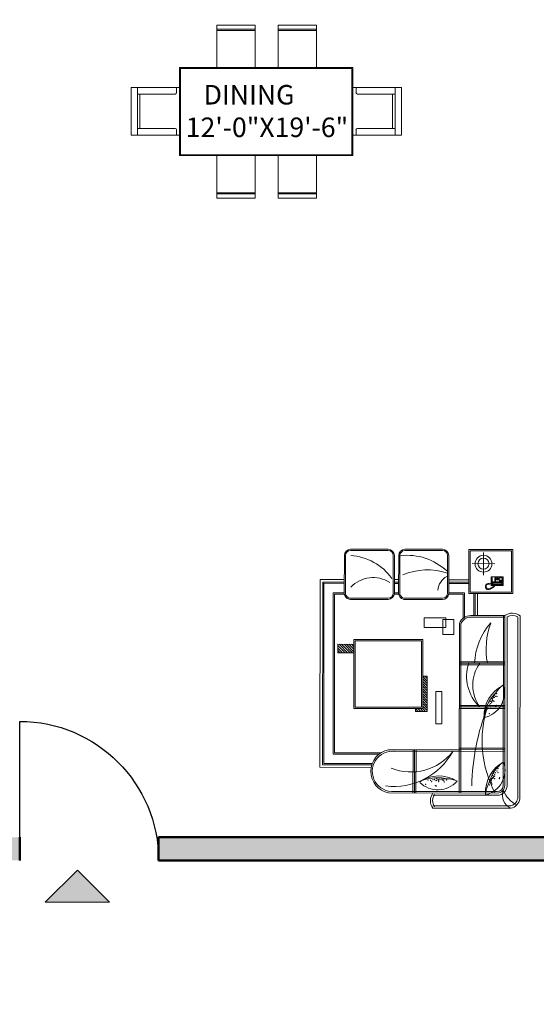
# Model space of a CAD drawing. Units: inches. Extents: x -7 to 1228, y -146 to 1091.
# Tile 49 of 88: x 242 to 376, y 531 to 786. Entities that reach past the tile are written whole.
import ezdxf

# ---------------------------------------------------------------- set-up
doc = ezdxf.new("R2010")
doc.units = ezdxf.units.IN
for name, color, linetype, lineweight in [('A-ANNO-SYMB', 30, 'Continuous', 18), ('A-AREA-IDEN', 7, 'Continuous', 18), ('A-DOOR', 4, 'Continuous', 25), ('A-FURN', 8, 'Continuous', 18), ('A-WALL', 7, 'Continuous', 50), ('A-WALL-PATT', 251, 'Continuous', 13)]:
    doc.layers.add(name, color=color, linetype=linetype, lineweight=lineweight)
doc.styles.get("Standard").update_dxf_attribs({"font": 'arial.ttf'})

# ---------------------------------------------------------------- blocks, each defined once
blk = doc.blocks.new('A$C317A697B')
for p, q in [((-116, 441), (-514, 441)), ((-514, 441), (-514, 0)), ((-116, 0), (-116, 441)), ((523, 441), (125, 441)), ((125, 441), (125, 0)), ((523, 0), (523, 441)), ((-116, 398), (-514, 398)), ((-116, 385), (-514, 385)), ((523, 398), (125, 398)), ((523, 385), (125, 385)), ((-899, -912), (-899, 0)), ((-899, 0), (899, 0)), ((899, 0), (899, -912)), ((-889, -902), (-889, -10)), ((-889, -10), (889, -10)), ((889, -10), (889, -902)), ((-899, -205), (-1402, -205)), ((-1402, -205), (-1402, -699)), ((-1336, -205), (-1336, -699)), ((-946, -274), (-1336, -274)), ((-1311, -274), (-1311, -630)), ((-932, -205), (-932, -259)), ((899, -205), (1402, -205)), ((932, -205), (932, -259)), ((946, -274), (1336, -274)), ((1311, -274), (1311, -630)), ((1336, -205), (1336, -699)), ((1402, -205), (1402, -699)), ((-1402, -699), (-899, -699)), ((-946, -630), (-1336, -630)), ((-932, -699), (-932, -645)), ((1402, -699), (899, -699)), ((932, -699), (932, -645)), ((946, -630), (1336, -630)), ((899, -912), (-899, -912)), ((889, -902), (-889, -902)), ((-514, -1353), (-514, -912)), ((-116, -912), (-116, -1353)), ((125, -1353), (125, -912)), ((523, -912), (523, -1353)), ((-116, -1297), (-514, -1297)), ((-116, -1309), (-514, -1309)), ((523, -1297), (125, -1297)), ((523, -1309), (125, -1309)), ((-116, -1353), (-514, -1353)), ((523, -1353), (125, -1353))]:
    blk.add_line(p, q)
for centre, start, end in [((-946, -259), 270, 0), ((946, -259), 180, 270), ((-946, -645), 0, 90), ((946, -645), 90, 180)]:
    blk.add_arc(centre, 14.7, start, end)
blk = doc.blocks.new('A$C327A19D4')
for p, q in [((1059, 3191), (3976, 3191)), ((1078, 3155), (3976, 3155)), ((703, 3073), (3, 3073)), ((3, 3073), (3, 2373)), ((683, 3053), (23, 3053)), ((23, 3053), (23, 2393)), ((683, 2393), (683, 3053)), ((703, 2373), (703, 3073)), ((1076, 2985), (3780, 2985)), ((4090, 3043), (4090, 1800)), ((4126, 3043), (4126, 1800)), ((1056, 2949), (3763, 2949)), ((1056, 2403), (1056, 2949)), ((1056, 2925), (3763, 2925)), ((1080, 2403), (1080, 2949)), ((1791, 2223), (1791, 2949)), ((1815, 2465), (1815, 2949)), ((1815, 2223), (1815, 2872)), ((1815, 2223), (1815, 2872)), ((1815, 2465), (1815, 2872)), ((1815, 2465), (1815, 2872)), ((1839, 2223), (1839, 2949)), ((2487, 2223), (2487, 2949)), ((2511, 2223), (2511, 2949)), ((2535, 2223), (2535, 2949)), ((3169, 2223), (3169, 2949)), ((3193, 2465), (3193, 2949)), ((3193, 2223), (3193, 2872)), ((3193, 2223), (3193, 2872)), ((3193, 2465), (3193, 2872)), ((3193, 2465), (3193, 2872)), ((3221, 1195), (3221, 2949)), ((3860, 2828), (3860, 1185)), ((3884, 2828), (3884, 1095)), ((3920, 2867), (3920, 1802)), ((231, 2784), (227, 2425)), ((49, 2607), (409, 2603)), ((703, 2512), (1056, 2512)), ((3, 2373), (703, 2373)), ((23, 2393), (683, 2393)), ((484, 2052), (484, 2373)), ((524, 2052), (524, 2373)), ((544, 2052), (544, 2373)), ((703, 2472), (1056, 2472)), ((703, 2452), (1056, 2452)), ((694, 2052), (694, 2302)), ((694, 2302), (1084, 2302)), ((714, 2051), (714, 2282)), ((714, 2282), (1098, 2282)), ((3884, 2247), (1184, 2247)), ((3884, 2223), (1184, 2223)), ((3195, 2235), (3195, 1095)), ((1119, 2135), (1357, 2135)), ((1119, 1958), (1119, 2135)), ((1357, 2135), (1357, 1958)), ((1092, 2007), (1244, 2007)), ((1092, 1659), (1092, 2007)), ((1357, 1958), (1119, 1958)), ((1244, 2007), (1244, 1659)), ((2265, 1945), (2780, 1945)), ((2265, 1845), (2265, 1945)), ((2780, 1945), (2780, 1845)), ((2780, 1845), (2265, 1845)), ((1244, 1659), (1092, 1659)), ((2539, 1638), (1439, 1638)), ((1439, 1638), (1439, 538)), ((2519, 1618), (1459, 1618)), ((1459, 1618), (1459, 558)), ((2023, 1638), (2023, 1711)), ((2023, 1711), (2585, 1711)), ((2519, 558), (2519, 1618)), ((2539, 538), (2539, 1638)), ((2585, 1711), (2585, 1522)), ((2585, 1522), (2539, 1522)), ((3884, 1532), (3195, 1532)), ((3884, 1508), (3195, 1508)), ((3884, 1484), (3195, 1484)), ((484, 1185), (484, 1252)), ((524, 1185), (524, 1252)), ((544, 1185), (544, 1252)), ((694, 1185), (694, 1252)), ((714, 1184), (714, 1253)), ((3247, 967), (3247, 230)), ((3267, 940), (3267, 210)), ((3417, 832), (3417, 60)), ((3437, 825), (3437, 40)), ((3477, 816), (3477, 0)), ((1439, 538), (2539, 538)), ((1459, 558), (2519, 558)), ((1516, 538), (1651, 538)), ((1516, 285), (1516, 538)), ((1651, 538), (1651, 285)), ((484, 0), (484, 385)), ((524, 40), (524, 385)), ((544, 60), (544, 385)), ((694, 210), (694, 385)), ((714, 230), (714, 386)), ((3267, 210), (694, 210)), ((3247, 230), (714, 230)), ((1651, 285), (1516, 285)), ((3437, 40), (524, 40)), ((3417, 60), (544, 60)), ((3477, 0), (484, 0))]:
    blk.add_line(p, q)
at = {"linetype": 'ByBlock'}
for p, q in [((438, 2915), (440, 2918)), ((439, 2728), (438, 2915)), ((440, 2918), (576, 2919)), ((451, 2906), (490, 2906)), ((451, 2856), (451, 2906)), ((491, 2856), (451, 2856)), ((453, 2831), (453, 2839)), ((453, 2839), (461, 2839)), ((461, 2831), (453, 2831)), ((461, 2839), (461, 2831)), ((466, 2839), (475, 2840)), ((467, 2831), (466, 2839)), ((475, 2831), (467, 2831)), ((475, 2840), (475, 2831)), ((480, 2840), (488, 2840)), ((480, 2831), (480, 2840)), ((488, 2832), (480, 2831)), ((488, 2840), (488, 2832)), ((490, 2906), (491, 2856)), ((505, 2903), (494, 2903)), ((494, 2903), (494, 2899)), ((494, 2899), (505, 2899)), ((495, 2895), (495, 2891)), ((505, 2895), (495, 2895)), ((495, 2891), (505, 2891)), ((495, 2887), (495, 2883)), ((505, 2887), (495, 2887)), ((495, 2883), (505, 2883)), ((495, 2879), (495, 2875)), ((505, 2879), (495, 2879)), ((495, 2875), (505, 2875)), ((495, 2871), (495, 2867)), ((506, 2871), (495, 2871)), ((495, 2867), (506, 2867)), ((495, 2863), (495, 2859)), ((506, 2863), (495, 2863)), ((495, 2859), (506, 2859)), ((505, 2899), (505, 2903)), ((505, 2891), (505, 2895)), ((505, 2883), (505, 2887)), ((505, 2875), (505, 2879)), ((506, 2867), (506, 2871)), ((506, 2859), (506, 2863)), ((515, 2908), (520, 2914)), ((516, 2744), (515, 2908)), ((520, 2910), (519, 2905)), ((519, 2905), (531, 2893)), ((519, 2905), (519, 2868)), ((519, 2868), (522, 2862)), ((520, 2914), (561, 2915)), ((526, 2913), (520, 2910)), ((522, 2862), (526, 2855)), ((532, 2895), (526, 2913)), ((526, 2913), (558, 2913)), ((526, 2855), (527, 2845)), ((527, 2845), (527, 2832)), ((528, 2806), (527, 2832)), ((531, 2893), (532, 2895)), ((532, 2832), (531, 2893)), ((551, 2896), (532, 2895)), ((532, 2832), (532, 2759)), ((551, 2896), (558, 2913)), ((553, 2893), (551, 2896)), ((565, 2905), (553, 2893)), ((553, 2832), (553, 2893)), ((553, 2832), (554, 2759)), ((558, 2855), (557, 2846)), ((557, 2846), (557, 2832)), ((557, 2806), (557, 2832)), ((558, 2913), (563, 2911)), ((562, 2862), (558, 2855)), ((561, 2915), (568, 2908)), ((565, 2869), (562, 2862)), ((563, 2911), (565, 2905)), ((565, 2905), (565, 2869)), ((568, 2908), (569, 2745)), ((576, 2919), (578, 2916)), ((578, 2916), (580, 2729)), ((442, 2726), (439, 2728)), ((543, 2726), (442, 2726)), ((453, 2824), (461, 2825)), ((453, 2816), (453, 2824)), ((461, 2816), (453, 2816)), ((453, 2801), (453, 2810)), ((453, 2810), (461, 2810)), ((461, 2802), (453, 2801)), ((453, 2787), (453, 2795)), ((453, 2795), (461, 2795)), ((461, 2787), (453, 2787)), ((468, 2743), (455, 2743)), ((455, 2743), (455, 2735)), ((455, 2735), (469, 2735)), ((461, 2825), (461, 2816)), ((461, 2810), (461, 2802)), ((461, 2795), (461, 2787)), ((467, 2816), (467, 2825)), ((467, 2825), (475, 2825)), ((475, 2817), (467, 2816)), ((467, 2802), (467, 2810)), ((467, 2810), (475, 2810)), ((475, 2802), (467, 2802)), ((467, 2787), (467, 2795)), ((467, 2795), (475, 2795)), ((475, 2787), (467, 2787)), ((469, 2735), (468, 2743)), ((487, 2743), (474, 2743)), ((474, 2743), (474, 2735)), ((474, 2735), (487, 2735)), ((475, 2825), (475, 2817)), ((475, 2810), (475, 2802)), ((475, 2795), (475, 2787)), ((480, 2817), (480, 2825)), ((480, 2825), (488, 2825)), ((488, 2817), (480, 2817)), ((480, 2810), (488, 2810)), ((480, 2802), (480, 2810)), ((488, 2802), (480, 2802)), ((480, 2787), (480, 2795)), ((480, 2795), (488, 2795)), ((488, 2787), (480, 2787)), ((487, 2735), (487, 2743)), ((488, 2825), (488, 2817)), ((488, 2810), (488, 2802)), ((488, 2795), (488, 2787)), ((493, 2744), (493, 2735)), ((506, 2744), (493, 2744)), ((493, 2735), (506, 2735)), ((497, 2795), (507, 2795)), ((497, 2787), (497, 2795)), ((507, 2787), (497, 2787)), ((506, 2735), (506, 2744)), ((507, 2795), (507, 2787)), ((523, 2737), (516, 2744)), ((520, 2783), (522, 2790)), ((520, 2746), (520, 2783)), ((520, 2746), (532, 2759)), ((521, 2741), (520, 2746)), ((527, 2738), (521, 2741)), ((522, 2790), (526, 2797)), ((542, 2737), (523, 2737)), ((526, 2797), (528, 2806)), ((533, 2756), (527, 2738)), ((527, 2738), (542, 2738)), ((532, 2759), (533, 2756)), ((552, 2756), (533, 2756)), ((546, 2743), (542, 2743)), ((542, 2743), (542, 2731)), ((542, 2731), (545, 2717)), ((545, 2717), (549, 2704)), ((547, 2732), (546, 2743)), ((546, 2738), (559, 2739)), ((562, 2737), (546, 2737)), ((549, 2696), (546, 2692)), ((546, 2692), (546, 2686)), ((546, 2686), (554, 2685)), ((554, 2685), (546, 2680)), ((546, 2680), (547, 2672)), ((548, 2723), (547, 2732)), ((547, 2672), (555, 2672)), ((577, 2726), (548, 2726)), ((552, 2710), (548, 2723)), ((549, 2704), (548, 2697)), ((548, 2697), (549, 2696)), ((555, 2672), (548, 2666)), ((554, 2759), (552, 2756)), ((552, 2756), (559, 2739)), ((553, 2703), (552, 2710)), ((552, 2696), (553, 2703)), ((557, 2693), (552, 2696)), ((566, 2747), (554, 2759)), ((556, 2687), (557, 2693)), ((558, 2669), (556, 2687)), ((559, 2797), (557, 2806)), ((568, 2656), (558, 2669)), ((563, 2790), (559, 2797)), ((559, 2739), (565, 2741)), ((569, 2745), (562, 2737)), ((566, 2783), (563, 2790)), ((565, 2741), (566, 2747)), ((566, 2747), (566, 2783)), ((580, 2729), (577, 2726)), ((587, 2779), (579, 2779)), ((579, 2775), (584, 2774)), ((584, 2774), (587, 2772)), ((590, 2777), (587, 2779)), ((587, 2772), (591, 2770)), ((594, 2771), (590, 2777)), ((591, 2770), (593, 2768)), ((595, 2768), (592, 2765)), ((592, 2765), (597, 2757)), ((593, 2768), (595, 2768)), ((599, 2771), (594, 2771)), ((597, 2757), (606, 2742)), ((602, 2770), (599, 2771)), ((599, 2760), (603, 2767)), ((606, 2763), (599, 2760)), ((603, 2767), (602, 2770)), ((604, 2750), (608, 2758)), ((612, 2753), (604, 2750)), ((608, 2758), (606, 2763)), ((606, 2742), (612, 2731)), ((608, 2742), (614, 2749)), ((615, 2746), (608, 2742)), ((614, 2749), (612, 2753)), ((612, 2731), (614, 2730)), ((613, 2733), (618, 2740)), ((621, 2736), (613, 2733)), ((614, 2730), (613, 2728)), ((613, 2728), (622, 2712)), ((618, 2740), (615, 2746)), ((620, 2723), (624, 2730)), ((627, 2725), (620, 2723)), ((624, 2730), (621, 2736)), ((622, 2712), (631, 2687)), ((626, 2712), (630, 2720)), ((634, 2713), (626, 2712)), ((630, 2720), (627, 2725)), ((631, 2687), (627, 2666)), ((628, 2702), (636, 2705)), ((637, 2702), (628, 2702)), ((631, 2672), (640, 2672)), ((638, 2665), (631, 2672)), ((633, 2691), (639, 2696)), ((641, 2691), (633, 2691)), ((636, 2705), (634, 2713)), ((634, 2681), (642, 2684)), ((641, 2677), (634, 2681)), ((639, 2696), (637, 2702)), ((640, 2672), (641, 2677)), ((642, 2684), (641, 2691)), ((548, 2666), (551, 2659)), ((551, 2659), (560, 2661)), ((560, 2661), (556, 2653)), ((556, 2653), (560, 2648)), ((560, 2648), (566, 2653)), ((566, 2653), (565, 2646)), ((565, 2646), (570, 2642)), ((583, 2649), (568, 2656)), ((570, 2642), (577, 2648)), ((577, 2648), (576, 2639)), ((576, 2639), (582, 2637)), ((582, 2637), (585, 2645)), ((599, 2647), (583, 2649)), ((585, 2645), (589, 2637)), ((589, 2637), (593, 2637)), ((593, 2637), (595, 2645)), ((595, 2645), (598, 2636)), ((598, 2636), (604, 2637)), ((615, 2654), (599, 2647)), ((604, 2645), (610, 2639)), ((604, 2637), (604, 2645)), ((610, 2639), (615, 2642)), ((614, 2650), (619, 2643)), ((615, 2642), (614, 2650)), ((627, 2666), (615, 2654)), ((619, 2643), (624, 2647)), ((620, 2654), (628, 2651)), ((624, 2647), (620, 2654)), ((628, 2661), (636, 2659)), ((632, 2654), (628, 2661)), ((628, 2651), (632, 2654)), ((636, 2659), (638, 2665))]:
    blk.add_line(p, q, dxfattribs=at)
at = {"ltscale": 5}
for p, q in [((100, 2052), (700, 2052)), ((0, 1352), (0, 1952)), ((20, 1352), (20, 1952)), ((100, 2032), (700, 2032)), ((780, 1952), (780, 1352)), ((800, 1952), (800, 1352)), ((2023, 1673), (2061, 1711)), ((2027, 1638), (2100, 1711)), ((2067, 1638), (2139, 1711)), ((2106, 1638), (2179, 1711)), ((2145, 1638), (2218, 1711)), ((2184, 1638), (2257, 1711)), ((2224, 1638), (2296, 1711)), ((2263, 1638), (2336, 1711)), ((2302, 1638), (2375, 1711)), ((2341, 1638), (2414, 1711)), ((2381, 1638), (2453, 1711)), ((2420, 1638), (2493, 1711)), ((2459, 1638), (2532, 1711)), ((2498, 1638), (2571, 1711)), ((2538, 1638), (2585, 1685)), ((2539, 1601), (2585, 1646)), ((2539, 1561), (2585, 1607)), ((2539, 1522), (2585, 1568)), ((2578, 1522), (2585, 1528)), ((700, 1272), (100, 1272)), ((700, 1252), (100, 1252)), ((100, 1185), (700, 1185)), ((100, 1165), (700, 1165)), ((0, 485), (0, 1085)), ((20, 485), (20, 1085)), ((780, 1085), (780, 485)), ((800, 1085), (800, 485)), ((1516, 499), (1555, 538)), ((1516, 460), (1594, 538)), ((1516, 421), (1634, 538)), ((1516, 382), (1651, 516)), ((1516, 342), (1651, 477)), ((700, 405), (100, 405)), ((700, 385), (100, 385)), ((1516, 303), (1651, 438)), ((1537, 285), (1651, 398)), ((1576, 285), (1651, 359)), ((1616, 285), (1651, 320))]:
    blk.add_line(p, q, dxfattribs=at)
for radius in [134, 88.7]:
    blk.add_circle((229, 2605), radius)
for centre, radius, start, end in [((1218, 3068), 201, 142.4201, 216.3682), ((1218, 3068), 165, 148.4003, 210.2229), ((3657, 3353), 468, 293.6733, 332.9672), ((3943, 3007), 150, 10.9855, 79.893), ((3943, 3007), 187, 10.9855, 79.893), ((3763, 2828), 157, 0, 90), ((3921, 3138), 226, 250.4844, 335.1673), ((2545, 3192), 468, 214.7097, 257.8799), ((2283, 2531), 409, 13.4523, 105.9639), ((2657, 3163), 547, 207.1715, 271.8037), ((3869, 3188), 547, 208.8478, 273.48), ((3911, 3323), 657, 217.6007, 253.5739), ((3517, 2544), 409, 14.6876, 107.1992), ((3763, 2828), 121, 0, 90), ((3763, 2828), 96.8, 0, 90), ((1594, 3859), 1211, 249.7283, 280.5443), ((1853, 3485), 1021, 228.2765, 267.8541), ((2752, 3267), 657, 227.0776, 263.0508), ((3052, 4350), 1764, 252.1519, 298.1592), ((3865, 6197), 3777, 248.9971, 268.5461), ((3951, 3106), 468, 222.7716, 265.9418), ((2024, 3008), 670, 251.8392, 316.629), ((2163, 3036), 599, 234.5154, 305.4846), ((1243, 2401), 187, 179.2584, 251.6848), ((1243, 2401), 163, 179.2584, 251.6848), ((4159, 1898), 547, 149.1529, 213.7851), ((4124, 2008), 468, 156.691, 199.8613), ((3425, 1881), 409, 315.4337, 47.9453), ((4298, 1873), 657, 169.059, 205.0321), ((4007, 1962), 201, 232.4201, 306.3682), ((4007, 1962), 165, 232.4201, 306.3682)]:
    blk.add_arc(centre, radius, start, end)
for centre, radius, start, end in [((100, 1952), 100, 90, 180), ((700, 1952), 100, 0, 90), ((100, 1952), 80, 90, 180), ((1024, 1388), 928, 137.1341, 186.5635), ((1307, 1706), 979, 160.9364, 203.1944), ((676, 2156), 279, 209.1633, 264.4137), ((700, 1952), 80, 0, 90), ((100, 1352), 100, 180, 270), ((100, 1352), 80, 180, 270), ((700, 1352), 80, 270, 0), ((700, 1352), 100, 270, 0), ((100, 1085), 100, 90, 180), ((100, 1085), 80, 90, 180), ((968, 436), 868, 125.4807, 176.5616), ((949, 846), 497, 147.8484, 226.1244), ((700, 1085), 100, 0, 90), ((700, 1085), 80, 0, 90), ((100, 485), 100, 180, 270), ((100, 485), 80, 180, 270), ((700, 485), 100, 270, 0), ((700, 485), 80, 270, 0)]:
    blk.add_arc(centre, radius, start, end, dxfattribs=at)
at = {"ltscale": 20}
for centre, radius, start, end in [((2701, 1449), 849, 338.2682, 52.2695), ((2703, 1175), 1078, 353.1988, 61.2564), ((3540, 1156), 321, 172.9078, 5.2194), ((3540, 1161), 351, 190.8398, 349.1602)]:
    blk.add_arc(centre, radius, start, end, dxfattribs=at)
for p in [(3492, 2920), (3495, 2842), (3560, 2838), (3641, 2868), (3657, 2862), (2298, 2818), (2329, 2780), (2344, 2802), (2345, 2825), (2356, 2781), (2375, 2736), (2410, 2757), (2421, 2774), (2421, 2720), (2444, 2738), (2445, 2691), (2459, 2715), (2481, 2700), (2485, 2814), (2498, 2803), (2514, 2718), (2515, 2690), (2620, 2701), (3535, 2825), (3561, 2800), (3571, 2765), (3585, 2789), (3609, 2758), (3612, 2788), (3646, 2728), (3647, 2768), (3655, 2787), (3694, 2735), (3707, 2710), (3719, 2734), (3738, 2747), (3756, 2703), (2551, 2664), (3648, 1911), (3660, 1974), (3676, 1951), (3677, 2020), (3684, 1893), (3687, 1973), (3705, 1892), (3707, 1984), (3646, 1828), (3658, 1864), (3673, 1803), (3674, 1829), (3683, 1768), (3686, 1853), (3706, 1784), (3770, 1842), (3772, 1859), (3680, 1724), (3748, 1685)]:
    blk.add_point(p)
blk = doc.blocks.new('DOOR-900')
blk.add_line((36, 0), (36, 36))
blk.add_arc((36, 0), 36, 90, 180)

msp = doc.modelspace()

# ---------------------------------------------------------------- hatches: boundary and pattern name
at = {"layer": 'A-ANNO-SYMB'}
h = msp.add_hatch(color=256, dxfattribs=at)
h.dxf.hatch_style = 1
h.paths.add_polyline_path([(256.95, 565.53), (248.61, 557.2), (265.29, 557.2)])
at = {"layer": 'A-WALL-PATT'}
h = msp.add_hatch(color=256, dxfattribs=at)
h.dxf.hatch_style = 1
h.paths.add_polyline_path([(69, 568), (60, 568), (60, 493), (63.29, 493), (69, 493)])
h.paths.add_polyline_path([(69, 662.41), (60, 662.41), (60, 586), (69, 586)], flags=17)
h.paths.add_polyline_path([(69, 723), (184, 723), (184, 734), (179, 734), (179, 728), (69, 728), (69, 741.62), (60, 741.62), (60, 698.41), (69, 698.41)], flags=17)
h.paths.add_polyline_path([(69, 782), (231, 782), (231, 728), (231, 723), (231, 586), (236, 586), (236, 787), (69, 787), (69, 800.13), (60, 800.13), (60, 765.62), (69, 765.62)])
h.paths.add_polyline_path([(184, 842), (189, 842), (189, 848), (173, 848), (173, 842), (179, 842), (179, 787), (184, 787)])
h.paths.add_polyline_path([(118.22, 69), (69, 69), (69, 60), (118.22, 60)])
h.paths.add_polyline_path([(227, 69), (154.22, 69), (154.22, 60), (227, 60)])
h.paths.add_polyline_path([(236, 60), (232.71, 60), (227, 60), (227, 36), (236, 36)])
h.paths.add_polyline_path([(389, 60), (380, 60), (380, 36), (389, 36)])
h.paths.add_polyline_path([(384, 181), (380, 181), (380, 115), (380, 78), (384, 78)])
h.paths.add_polyline_path([(380, 115), (334.55, 115), (334.55, 109), (380, 109)])
h.paths.add_polyline_path([(274.55, 115), (236, 115), (236, 201), (232.71, 201), (231, 201), (231, 78), (236, 78), (236, 109), (274.55, 109)])
h.paths.add_polyline_path([(69, 123), (60, 123), (60, 78), (69, 78)])
h.paths.add_polyline_path([(69, 201), (60, 201), (60, 159), (69, 159)])
h.paths.add_polyline_path([(143, 219), (69, 219), (69, 213), (143, 213)], flags=17)
h.paths.add_polyline_path([(189, 219), (184, 219), (184, 274), (231, 274), (231, 219), (236, 219), (236, 279), (184, 279), (184, 297), (179, 297), (179, 279), (69, 279), (69, 290.91), (60, 290.91), (60, 262.18), (69, 262.18), (69, 274), (179, 274), (179, 219), (173, 219), (173, 213), (189, 213)])
h.paths.add_polyline_path([(69, 238.18), (60, 238.18), (60, 219), (69, 219)], flags=17)
h.paths.add_polyline_path([(69, 333), (60, 333), (60, 314.91), (69, 314.91), (69, 316.96)])
h.paths.add_polyline_path([(190, 338), (184, 338), (69, 338), (69, 333), (179, 333), (179, 327), (184, 327), (184, 333.02), (190, 333.05)])
h.paths.add_polyline_path([(69, 386.81), (60, 386.81), (60, 351), (69, 351)])
h.paths.add_polyline_path([(69, 475), (60, 475), (60, 422.81), (69, 422.81)])
h.paths.add_polyline_path([(236, 475), (231, 475), (231, 351.24), (236, 351.24)])
h.paths.add_polyline_path([(384, 475), (380, 475), (380, 362), (384, 362)])
h.paths.add_polyline_path([(547, 307), (439, 307), (439, 356), (445, 356), (445, 362), (433, 362), (433, 307), (380, 307), (380, 244), (380, 241), (384, 241), (384, 301), (433, 301), (433, 277), (439, 277), (439, 301), (547, 301)])
h.paths.add_polyline_path([(547, 241), (439, 241), (439, 247), (433, 247), (433, 235), (547, 235)])
h.paths.add_polyline_path([(450, 69), (440.29, 69), (424.89, 69), (389, 69), (389, 60), (450, 60)])
h.paths.add_polyline_path([(547, 69), (486, 69), (486, 60), (547, 60)])
h.paths.add_polyline_path([(556, 148.27), (547, 148.27), (547, 78), (556, 78)])
h.paths.add_polyline_path([(556, 223), (547, 223), (547, 195), (547, 184.27), (556, 184.27)])
h.paths.add_polyline_path([(556, 311.19), (547, 311.19), (547, 273.08), (556, 273.08)])
h.paths.add_polyline_path([(556, 344), (552.71, 344), (547, 344), (547, 335.19), (556, 335.19)])
h.paths.add_polyline_path([(556, 249.08), (547, 249.08), (547, 241), (556, 241)])
h.paths.add_polyline_path([(547, 362), (475, 362), (475, 356), (547, 356)], flags=0)
h.paths.add_polyline_path([(556, 399.62), (547, 399.62), (547, 362), (556, 362)])
h.paths.add_polyline_path([(556, 475), (547, 475), (547, 435.62), (556, 435.62)])
h.paths.add_polyline_path([(547, 493), (389, 493), (389, 487), (547, 487)])
h.paths.add_polyline_path([(380, 493), (278, 493), (278, 487), (380, 487)])
h.paths.add_polyline_path([(227, 493), (69, 493), (69, 487), (227, 487)])
h.paths.add_polyline_path([(643, 122.44), (634, 122.44), (634, 78), (643, 78)])
h.paths.add_polyline_path([(702.5, 69), (692.79, 69), (677.39, 69), (643, 69), (643, 60), (702.5, 60)])
h.paths.add_polyline_path([(798, 69), (738.5, 69), (738.5, 60), (798, 60)])
h.paths.add_polyline_path([(807, 60), (803.71, 60), (798, 60), (798, 36), (807, 36)])
h.paths.add_polyline_path([(807, 109), (846.75, 109), (846.75, 115), (807, 115), (807, 159), (802, 159), (802, 78), (807, 78)])
h.paths.add_polyline_path([(807, 201), (802, 201), (802, 195), (807, 195)])
h.paths.add_polyline_path([(643, 201), (634, 201), (634, 158.44), (643, 158.44)])
h.paths.add_polyline_path([(756, 225), (751, 225), (751, 219), (643, 219), (643, 213), (756, 213)])
h.paths.add_polyline_path([(643, 240.85), (634, 240.85), (634, 219), (643, 219)])
h.paths.add_polyline_path([(643, 274), (643, 288.63), (634, 288.63), (634, 264.85), (643, 264.85)])
h.paths.add_polyline_path([(802, 279), (756, 279), (756, 297), (751, 297), (751, 279), (643, 279), (643, 274), (751, 274), (751, 255), (756, 255), (756, 274), (802, 274)])
h.paths.add_polyline_path([(807, 333), (803.71, 333), (802, 333), (802, 279), (802, 274), (802, 219), (807, 219)])
h.paths.add_polyline_path([(956, 182), (951, 182), (951, 115), (906.75, 115), (906.75, 109), (951, 109), (951, 78), (956, 78)])
h.paths.add_polyline_path([(960, 60), (951, 60), (951, 36), (960, 36)])
h.paths.add_polyline_path([(1021, 69), (1005.78, 69), (960, 69), (960, 60), (1021, 60)])
h.paths.add_polyline_path([(956, 224), (951, 224), (951, 218), (956, 218)])
h.paths.add_polyline_path([(956, 302), (1004, 302), (1004, 278), (1010, 278), (1010, 302), (1118, 302), (1118, 290.81), (1127, 290.81), (1127, 326.97), (1118, 326.97), (1118, 320.97), (1118, 307), (1010, 307), (1010, 356), (1016, 356), (1016, 362), (1004, 362), (1004, 307), (951, 307), (951, 244), (951, 242), (954.29, 242), (956, 242)])
h.paths.add_polyline_path([(643, 333), (634, 333), (634, 312.63), (643, 312.63), (643, 316.96)])
h.paths.add_polyline_path([(756, 338), (643, 338), (643, 333), (751, 333), (751, 327), (756, 327)])
h.paths.add_polyline_path([(643, 388), (634, 388), (634, 351), (643, 351)])
h.paths.add_polyline_path([(807, 357), (802, 357), (802, 351), (807, 351)])
h.paths.add_polyline_path([(807, 475), (802, 475), (802, 393), (807, 393)])
h.paths.add_polyline_path([(643, 475), (634, 475), (634, 424), (643, 424)])
h.paths.add_polyline_path([(798, 493), (643, 493), (643, 487), (798, 487)])
h.paths.add_polyline_path([(634, 493), (556, 493), (556, 487), (634, 487)])
h.paths.add_polyline_path([(813, 493), (807, 493), (807, 487), (813, 487)])
h.paths.add_polyline_path([(951, 493), (849, 493), (849, 487), (951, 487)])
h.paths.add_polyline_path([(956, 484), (951, 484), (951, 374), (956, 374)])
h.paths.add_polyline_path([(1109, 493), (969, 493), (969, 487), (1109, 487)])
h.paths.add_polyline_path([(1127, 484), (1118, 484), (1118, 450.64), (1127, 450.64)])
h.paths.add_polyline_path([(1127, 414.64), (1118, 414.64), (1118, 365), (1127, 365)])
h.paths.add_polyline_path([(1109, 362), (1046, 362), (1046, 356), (1109, 356)], flags=17)
h.paths.add_polyline_path([(1127, 356), (1123.45, 356), (1118, 356), (1118, 350.97), (1127, 350.97)], flags=0)
h.paths.add_polyline_path([(1127, 266.81), (1118, 266.81), (1118, 262.36), (1118, 242), (1127, 242)], flags=17)
h.paths.add_polyline_path([(1118, 242), (1010, 242), (1010, 248), (1004, 248), (1004, 237), (1118, 237)])
h.paths.add_polyline_path([(1127, 224), (1118, 224), (1118, 170), (1127, 170)])
h.paths.add_polyline_path([(1127, 134), (1118, 134), (1118, 78), (1127, 78)])
h.paths.add_polyline_path([(1118, 69), (1057, 69), (1057, 60), (1118, 60)])
h.paths.add_polyline_path([(227, 571.55), (227, 574), (69, 574), (69, 568), (227, 568)])
h.paths.add_polyline_path([(380, 571.55), (380, 574), (278, 574), (278, 568), (380, 568)])
h.paths.add_polyline_path([(242, 574), (236, 574), (236, 568), (242, 568)])
h.paths.add_polyline_path([(547, 571.55), (547, 574), (389, 574), (389, 568), (547, 568)])
h.paths.add_polyline_path([(384, 733), (380, 733), (380, 586), (384, 586)])
h.paths.add_polyline_path([(556, 646), (634, 646), (634, 655), (547, 655), (547, 586), (556, 586)])
h.paths.add_polyline_path([(634, 574), (556, 574), (556, 568), (634, 568)])
h.paths.add_polyline_path([(643, 655), (634, 655), (634, 586), (643, 586)])
h.paths.add_polyline_path([(798, 574), (643, 574), (643, 568), (798, 568)])
h.paths.add_polyline_path([(643, 663.85), (634, 663.85), (634, 655), (643, 655)])
h.paths.add_polyline_path([(556, 676.97), (547, 676.97), (547, 655), (556, 655)])
h.paths.add_polyline_path([(556, 733), (547, 733), (547, 712.97), (556, 712.97)])
h.paths.add_polyline_path([(643, 710), (634, 710), (634, 699.85), (643, 699.85)])
h.paths.add_polyline_path([(807, 668), (802, 668), (802, 586), (807, 586)])
h.paths.add_polyline_path([(951, 574), (849, 574), (849, 568), (951, 568)])
h.paths.add_polyline_path([(956, 691), (951, 691), (951, 577), (956, 577)])
h.paths.add_polyline_path([(1109, 574), (969, 574), (969, 568), (1109, 568)])
h.paths.add_polyline_path([(1127, 643.4), (1118, 643.4), (1118, 577), (1127, 577)])
h.paths.add_polyline_path([(1127, 568), (1123.45, 568), (1118, 568), (1118, 493), (1127, 493)])
h.paths.add_polyline_path([(1127, 733), (1118, 733), (1118, 679.4), (1127, 679.4)])
h.paths.add_polyline_path([(1127, 777.35), (1118, 777.35), (1118, 770.04), (1118, 751), (1127, 751)], flags=17)
h.paths.add_polyline_path([(1118, 751), (1010, 751), (1010, 757), (1004, 757), (1004, 745), (1118, 745)])
h.paths.add_polyline_path([(956, 811), (1004, 811), (1004, 787), (1010, 787), (1010, 811), (1017.87, 811), (1017.87, 811.63, -0.414214), (1018.25, 812), (1031.98, 812, -0.414214), (1032.35, 811.63), (1032.35, 811), (1118, 811), (1118, 801.35), (1127, 801.35), (1127, 834.69), (1118, 834.69), (1118, 830.24), (1118, 817), (1010, 817), (1010, 866), (1016, 866), (1016, 872), (1004, 872), (1004, 817), (956, 817), (956, 866), (951, 866), (951, 751), (954.29, 751), (956, 751)])
h.paths.add_polyline_path([(1118, 872), (1046, 872), (1046, 866), (1118, 866)], flags=17)
h.paths.add_polyline_path([(1127, 924.71), (1118, 924.71), (1118, 884), (1127, 884)])
h.paths.add_polyline_path([(1127, 866), (1123.71, 866), (1118, 866), (1118, 858.69), (1127, 858.69)], flags=17)
h.paths.add_polyline_path([(956, 983), (951, 983), (951, 952), (807, 952), (807, 983), (802, 983), (802, 902), (807, 902), (807, 946), (951, 946), (951, 884), (956, 884)])
h.paths.add_polyline_path([(807, 842), (802, 842), (802, 787), (756, 787), (756, 806), (751, 806), (751, 787), (643, 787), (643, 782), (751, 782), (751, 764), (756, 764), (756, 782), (802, 782), (802, 728), (807, 728)])
h.paths.add_polyline_path([(756, 848), (643, 848), (643, 842), (751, 842), (751, 836), (756, 836)])
h.paths.add_polyline_path([(756, 734), (751, 734), (751, 728), (643, 728), (643, 723), (756, 723)])
h.paths.add_polyline_path([(643, 749.79), (634, 749.79), (634, 728), (637.29, 728), (643, 728)])
h.paths.add_polyline_path([(643, 805.41), (634, 805.41), (634, 773.79), (643, 773.79)])
h.paths.add_polyline_path([(643, 896.66), (634, 896.66), (634, 860), (637.29, 860), (643, 860)])
h.paths.add_polyline_path([(643, 842), (634, 842), (634, 829.41), (643, 829.41)])
h.paths.add_polyline_path([(643, 983), (634, 983), (634, 932.66), (643, 932.66)])
h.paths.add_polyline_path([(1127, 983), (1118, 983), (1118, 960.71), (1127, 960.71)])
h.paths.add_polyline_path([(1118, 1001), (1077.53, 1001), (1077.53, 992), (1118, 992)])
h.paths.add_polyline_path([(1041.53, 1001), (960, 1001), (960, 992), (1041.53, 992)])
h.paths.add_polyline_path([(960, 1025), (951, 1025), (951, 1001), (954.29, 1001), (960, 1001)])
h.paths.add_polyline_path([(807, 1025), (798, 1025), (798, 1001), (807, 1001)])
h.paths.add_polyline_path([(798, 1001), (738.5, 1001), (738.5, 992), (798, 992)])
h.paths.add_polyline_path([(702.5, 1001), (643, 1001), (643, 992), (702.5, 992)])
h.paths.add_polyline_path([(547, 1001), (499.11, 1001), (499.11, 992), (547, 992)])
h.paths.add_polyline_path([(463.11, 1001), (389, 1001), (389, 992), (463.11, 992)])
h.paths.add_polyline_path([(389, 1025), (380, 1025), (380, 1022), (380, 1001), (383.29, 1001), (389, 1001)])
h.paths.add_polyline_path([(236, 1025), (227, 1025), (227, 1001), (236, 1001)])
h.paths.add_polyline_path([(236, 983), (231, 983), (231, 860), (236, 860)])
h.paths.add_polyline_path([(274.55, 952), (236, 952), (236, 946), (274.55, 946)])
h.paths.add_polyline_path([(380, 952), (334.55, 952), (334.55, 946), (380, 946)])
h.paths.add_polyline_path([(384, 983), (380, 983), (380, 884), (383.29, 884), (384, 884)])
h.paths.add_polyline_path([(227, 1001), (155.01, 1001), (155.01, 992), (162.87, 992), (227, 992)])
h.paths.add_polyline_path([(119.01, 1001), (69, 1001), (69, 992), (119.01, 992)])
h.paths.add_polyline_path([(69, 983), (60, 983), (60, 922.99), (69, 922.99)])
h.paths.add_polyline_path([(69, 886.99), (60, 886.99), (60, 860), (63.29, 860), (69, 860)])
h.paths.add_polyline_path([(143, 848), (69, 848), (69, 842), (143, 842)])

# ---------------------------------------------------------------- linework, layer by layer
at = {"layer": 'A-ANNO-SYMB'}
for p, q in [((256.95, 565.53), (248.61, 557.2)), ((256.95, 565.53), (265.29, 557.2)), ((248.61, 557.2), (265.29, 557.2))]:
    msp.add_line(p, q, dxfattribs=at)
at = {"layer": 'A-WALL'}
for p, q in [((242, 574), (242, 568)), ((278, 574), (278, 568)), ((380, 574), (278, 574)), ((380, 568), (278, 568))]:
    msp.add_line(p, q, dxfattribs=at)

# ---------------------------------------------------------------- block references
at = {"layer": 'A-DOOR', "extrusion": (0, 0, -1), "zscale": -1}
msp.add_blockref('DOOR-900', (-278, 568), dxfattribs=at)
at = {"layer": 'A-FURN', "xscale": 0.024965713951469, "yscale": 0.024965713951469, "zscale": 0.024965713951469}
msp.add_blockref('A$C317A697B', (305.87, 773.19), dxfattribs=at)
at = {"layer": 'A-FURN', "xscale": 0.016235792481004, "yscale": 0.016235792481004, "zscale": 0.016235792481004, "rotation": 269.9431658144944}
msp.add_blockref('A$C327A19D4', (319.85, 648.56), dxfattribs=at)

# ---------------------------------------------------------------- texts
at = {"layer": 'A-AREA-IDEN', "insert": (285.02, 768.71), "char_height": 5.0568, "attachment_point": 1}
msp.add_mtext_dynamic_manual_height_columns('   DINING\\P12\'-0"X19\'-6"', width=137.2821, gutter_width=25.28, heights=[0], dxfattribs=at)

doc.saveas('drawing.dxf')
